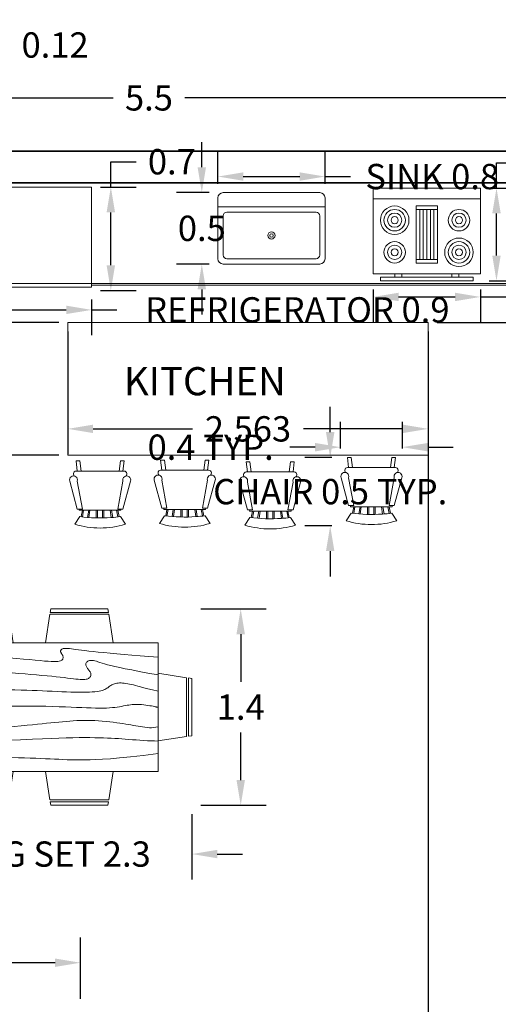
# Model space of a CAD drawing. Units: metres. Extents: x 4.8 to 18.3, y 28.2 to 89.8.
# Tile 3 of 4: x 8.6 to 12, y 36.6 to 43.6. Entities that reach past the tile are written whole.
import ezdxf

# ---------------------------------------------------------------- set-up
doc = ezdxf.new("R2010")
doc.units = ezdxf.units.M
doc.header["$MEASUREMENT"] = 0
doc.layers.get('Defpoints').update_dxf_attribs({"color": 3})
for name, color, linetype, lineweight in [('A-ANNO-DIMS', 2, 'Continuous', 18), ('A-AREA-IDEN', 7, 'Continuous', 25), ('A-EQPM', 8, 'Continuous', 18), ('A-FLOR-CASE', 8, 'Continuous', 18), ('A-FLOR-FIXT', 9, 'Continuous', 18), ('A-FURN', 8, 'Continuous', 18), ('A-WALL', 7, 'Continuous', 35)]:
    doc.layers.add(name, color=color, linetype=linetype, lineweight=lineweight)
doc.styles.get("Standard").update_dxf_attribs({"font": 'arial.ttf'})
doc.dimstyles.get("Standard").update_dxf_attribs({"dimtxt": 0.18, "dimasz": 0.18, "dimexe": 0.18, "dimexo": 0.0625, "dimgap": 0.09, "dimtad": 0, "dimtih": 1, "dimtoh": 1, "dimdec": 1, "dimzin": 0, "dimdsep": 46, "dimtxsty": 'Standard', "dimcen": 0.09, "dimadec": 0, "dimazin": 0, "dimtfac": 1, "dimtdec": 1, "dimtofl": 0, "dimtmove": 0, "dimatfit": 3, "dimfxl": 1, "dimtolj": 1, "dimtzin": 0, "dimarcsym": 0})

# ---------------------------------------------------------------- blocks, each defined once
blk = doc.blocks.new('Refrigerator-2 door - 36 in top')
for p, q in [((0, -26.999999), (36, -26.999999)), ((12, -26.999999), (12, -28.999999)), ((11, -27.999999), (11, -28.999999)), ((11, -28.999999), (13, -28.999999)), ((13, -28.999999), (13, -27.999999))]:
    blk.add_line(p, q)
blk.add_lwpolyline([(0, -27.999999), (0, 0), (36, 0), (36, -27.999999)], close=True)
blk = doc.blocks.new('Range-Oven - 30 in top')
for p, q in [((0, -3), (30, -3)), ((12, -6), (18, -6)), ((13, -20), (13, -6)), ((14, -6), (14, -20)), ((15, -20), (15, -6)), ((16, -6), (16, -20)), ((17, -20), (17, -6)), ((18, -20), (12, -20)), ((6, -24), (6, -25)), ((8, -25), (8, -24)), ((22, -25), (22, -24)), ((24, -24), (24, -25))]:
    blk.add_line(p, q)
for points in [[(0, -24), (0, 0), (30, 0), (30, -24)], [(12, -21), (12, -5), (18, -5), (18, -21)], [(2, -26), (2, -25), (28, -25), (28, -26)]]:
    blk.add_lwpolyline(points, close=True)
for centre, radius in [((6, -9), 4), ((6, -9), 3), ((6, -9), 2), ((6, -9), 1), ((24, -9), 3), ((24, -9), 2), ((24, -9), 1), ((6, -18), 3), ((6, -18), 2), ((24, -18), 4), ((24, -18), 3), ((24, -18), 2), ((6, -18), 1), ((24, -18), 1)]:
    blk.add_circle(centre, radius)
blk = doc.blocks.new('Sink-single - 30 in top')
blk.add_line((-15, -3.999996), (15, -3.999996))
for points in [[(-13.5, 0), (13.5, 0)], [(-15, -18.499996), (-15, -1.5)], [(15, -1.5), (15, -18.499996)], [(-12.5, -5.499996), (12.5, -5.499996)], [(-13.5, -17.499996), (-13.5, -6.499996)], [(13.5, -6.499996), (13.5, -17.499996)], [(12.5, -18.499996), (-12.5, -18.499996)], [(13.5, -19.999996), (-13.5, -19.999996)]]:
    blk.add_lwpolyline(points)
for radius in [1, 0.5]:
    blk.add_circle((0, -11.999996), radius)
for centre, radius, start, end in [((-13.5, -1.5), 1.5, 90, 180), ((13.5, -1.5), 1.5, 0, 90), ((-12.5, -6.499996), 1, 90, 180), ((12.5, -6.499996), 1, 0, 90), ((-13.5, -18.499996), 1.5, 180, 270), ((-12.5, -17.499996), 1, 180, 270), ((12.5, -17.499996), 1, 270, 0), ((13.5, -18.499996), 1.5, 270, 0)]:
    blk.add_arc(centre, radius, start, end)
blk = doc.blocks.new('Dining Set - 36 x 72 in.')
for p, q in [((-22.2343, 26.00059), (-23.4847, 17.99762)), ((-22.2304, 26), (-5.7608, 26)), ((-22, 27.5), (-22.1562, 26.50042)), ((-5.8416, 26.5), (-22.1534, 26.5)), ((-22, 27.5), (-6, 27.5)), ((-5.8437, 26.49966), (-6, 27.5)), ((-4.5152, 17.99762), (-5.7655, 25.99926)), ((5.7657, 26.00059), (4.5153, 17.99762)), ((5.7696, 26), (22.2392, 26)), ((6, 27.5), (5.8438, 26.50042)), ((22.1584, 26.5), (5.8466, 26.5)), ((6, 27.5), (22, 27.5)), ((22.1563, 26.49966), (22, 27.5)), ((23.4848, 17.99762), (22.2345, 25.99926)), ((36, 18), (-36, 18)), ((-36, 18), (-36, -18)), ((36, -18), (36, 18)), ((-44.0006, 8.23428), (-35.9976, 9.48474)), ((44.0006, 8.23428), (35.9976, 9.48474)), ((-45.5, 8), (-44.5004, 8.15617)), ((-45.5, 8), (-45.5, -8)), ((-44.5, -8.15843), (-44.5, 8.15338)), ((-44, 8.23041), (-44, -8.23915)), ((44, 8.23041), (44, -8.23915)), ((44.5, -8.15843), (44.5, 8.15338)), ((45.5, 8), (44.5005, 8.15617)), ((45.5, 8), (45.5, -8)), ((-44.4997, -8.15631), (-45.5, -8)), ((-35.9976, -9.48476), (-43.9993, -8.2345)), ((35.9976, -9.48476), (43.9993, -8.2345)), ((44.4997, -8.15631), (45.5, -8)), ((-36, -18), (36, -18)), ((-22.2343, -26.0006), (-23.4847, -17.99762)), ((-4.5152, -17.99762), (-5.7655, -25.99928)), ((5.7657, -26.0006), (4.5153, -17.99762)), ((23.4848, -17.99762), (22.2345, -25.99928)), ((-22.2304, -26), (-5.7608, -26)), ((-22, -27.5), (-22.1562, -26.50044)), ((-5.8416, -26.5), (-22.1534, -26.5)), ((-22, -27.5), (-6, -27.5)), ((-5.8437, -26.49967), (-6, -27.5)), ((5.7696, -26), (22.2392, -26)), ((6, -27.5), (5.8438, -26.50044)), ((22.1584, -26.5), (5.8466, -26.5)), ((6, -27.5), (22, -27.5)), ((22.1563, -26.49967), (22, -27.5))]:
    blk.add_line(p, q)
for points in [[(-36, 15), (-31.1772, 14.97754), (-26.8079, 14.91406), (-22.8538, 14.81543), (-19.276, 14.6875), (-16.0362, 14.53613), (-13.0957, 14.36718), (-10.4159, 14.18652), (-7.9583, 14), (-5.6904, 13.81315), (-3.6035, 13.63021), (-1.6954, 13.45508), (0.0365, 13.29166), (1.5945, 13.14388), (2.9811, 13.01562), (4.1988, 12.9108), (5.25, 12.83333), (6.1393, 12.78613), (6.8802, 12.76823), (7.4883, 12.77767), (7.9792, 12.8125), (8.3685, 12.87077), (8.6719, 12.95052), (8.9049, 13.0498), (9.0833, 13.16666), (9.2205, 13.29899), (9.3216, 13.44401), (9.3895, 13.59879), (9.4271, 13.76041), (9.4373, 13.92594), (9.4232, 14.09245), (9.3875, 14.257), (9.3333, 14.41666), (9.2638, 14.56917), (9.1836, 14.71484), (9.0975, 14.85465), (9.0104, 14.98958), (8.9272, 15.1206), (8.8529, 15.2487), (8.7922, 15.37483), (8.75, 15.5), (8.7305, 15.62467), (8.7344, 15.74739), (8.7617, 15.86621), (8.8125, 15.97916), (8.8867, 16.08431), (8.9844, 16.17968), (9.1055, 16.26334), (9.25, 16.33333), (9.4189, 16.38802), (9.6172, 16.42708), (9.8506, 16.45052), (10.125, 16.45833), (10.4463, 16.45052), (10.8203, 16.42708), (11.2529, 16.38802), (11.75, 16.33333), (12.3184, 16.26318), (12.9694, 16.17838), (13.7151, 16.07991), (14.5677, 15.96875), (15.5395, 15.84586), (16.6426, 15.71224), (17.8893, 15.56884), (19.2917, 15.41666), (20.859, 15.25667), (22.5879, 15.08984), (24.4721, 14.91715), (26.5052, 14.73958), (28.6809, 14.5581), (30.9929, 14.3737), (33.4347, 14.18733), (36, 14)], [(-36, 10), (-28.9766, 10.14274), (-23.1725, 10.20442), (-18.4241, 10.19775), (-14.5677, 10.13541), (-11.4399, 10.03011), (-8.877, 9.89453), (-6.7154, 9.74137), (-4.7917, 9.58333), (-2.9698, 9.43082), (-1.2246, 9.28515), (0.4415, 9.14534), (2.026, 9.01041), (3.5266, 8.87939), (4.9408, 8.7513), (6.266, 8.62516), (7.5, 8.5), (8.6411, 8.37549), (9.6914, 8.2539), (10.6538, 8.13818), (11.5312, 8.03125), (12.3267, 7.93603), (13.043, 7.85547), (13.6831, 7.79248), (14.25, 7.75), (14.7471, 7.7303), (15.1797, 7.73307), (15.5537, 7.75732), (15.875, 7.80208), (16.1494, 7.86637), (16.3828, 7.94922), (16.5811, 8.04964), (16.75, 8.16666), (16.8944, 8.29915), (17.0143, 8.44531), (17.1089, 8.60319), (17.1771, 8.77083), (17.218, 8.94629), (17.2305, 9.1276), (17.2137, 9.31282), (17.1667, 9.5), (17.0895, 9.6875), (16.987, 9.875), (16.8649, 10.0625), (16.7292, 10.25), (16.5856, 10.4375), (16.4401, 10.625), (16.2985, 10.8125), (16.1667, 11), (16.05, 11.18733), (15.9518, 11.3737), (15.8752, 11.5581), (15.8229, 11.73958), (15.798, 11.91715), (15.8034, 12.08984), (15.842, 12.25667), (15.9167, 12.41666), (16.0295, 12.56836), (16.1784, 12.70833), (16.3605, 12.83268), (16.5729, 12.9375), (16.8127, 13.01888), (17.0768, 13.07291), (17.3625, 13.0957), (17.6667, 13.08333), (17.9894, 13.03312), (18.3418, 12.94726), (18.7382, 12.82918), (19.1927, 12.68229), (19.7195, 12.51001), (20.3327, 12.31575), (21.0465, 12.10294), (21.875, 11.875), (22.8357, 11.63354), (23.959, 11.37304), (25.2786, 11.08618), (26.8282, 10.76562), (28.6414, 10.40405), (30.752, 9.99414), (33.1936, 9.52856), (36, 9)], [(-36, 5.5), (-30.7157, 5.3348), (-26.069, 5.20963), (-21.9946, 5.11767), (-18.4271, 5.05208), (-15.3009, 5.00602), (-12.5508, 4.97265), (-10.1112, 4.94515), (-7.9167, 4.91666), (-5.909, 4.88167), (-4.0586, 4.83984), (-2.3429, 4.79215), (-0.7396, 4.73958), (0.7739, 4.6831), (2.22, 4.6237), (3.6213, 4.56233), (5, 4.5), (6.373, 4.43782), (7.7344, 4.3776), (9.0723, 4.32129), (10.375, 4.27083), (11.6309, 4.22819), (12.8281, 4.19531), (13.9551, 4.17415), (15, 4.16666), (15.954, 4.17448), (16.819, 4.19791), (17.6001, 4.23698), (18.3021, 4.29166), (18.9299, 4.36198), (19.4883, 4.44791), (19.9823, 4.54948), (20.4167, 4.66666), (20.7969, 4.79899), (21.1302, 4.94401), (21.4245, 5.09879), (21.6875, 5.26041), (21.9271, 5.42594), (22.1511, 5.59245), (22.3672, 5.757), (22.5834, 5.91666), (22.8065, 6.06868), (23.0404, 6.21093), (23.2879, 6.34147), (23.5521, 6.45833), (23.8358, 6.55957), (24.142, 6.64323), (24.4735, 6.70735), (24.8334, 6.75), (25.2235, 6.76969), (25.642, 6.76692), (26.0858, 6.74267), (26.5521, 6.69791), (27.0379, 6.63362), (27.5404, 6.55078), (28.0565, 6.45036), (28.5834, 6.33333), (29.1242, 6.19987), (29.7071, 6.04687), (30.3661, 5.87044), (31.1354, 5.66666), (32.0493, 5.43164), (33.142, 5.16146), (34.4475, 4.85221), (36, 4.5)], [(-36, -1), (-30.7915, -0.6591), (-26.0195, -0.38216), (-21.6519, -0.16284), (-17.6563, 0.00521), (-14.0005, 0.12833), (-10.6523, 0.21289), (-7.5796, 0.26522), (-4.75, 0.29166), (-2.134, 0.29793), (0.2878, 0.28711), (2.5317, 0.26163), (4.6146, 0.22396), (6.5529, 0.17651), (8.3633, 0.12174), (10.0623, 0.06209), (11.6667, 0), (13.1899, -0.06201), (14.6341, -0.1211), (15.9982, -0.17432), (17.2813, -0.21875), (18.4823, -0.25147), (19.6003, -0.26953), (20.6343, -0.27002), (21.5834, -0.25), (22.4481, -0.20768), (23.2357, -0.14584), (23.9549, -0.06836), (24.6146, 0.02083), (25.2235, 0.11784), (25.7904, 0.21875), (26.3241, 0.31966), (26.8334, 0.41666), (27.3265, 0.50618), (27.8099, 0.58593), (28.2894, 0.65397), (28.7709, 0.70833), (29.2601, 0.74707), (29.763, 0.76823), (30.2855, 0.76985), (30.8334, 0.75), (31.4088, 0.70784), (31.9994, 0.64713), (32.589, 0.57275), (33.1615, 0.48958), (33.7008, 0.4025), (34.1908, 0.3164), (34.6153, 0.23616), (34.9584, 0.16666), (35.2099, 0.11165), (35.3848, 0.07031), (35.504, 0.04069), (35.5886, 0.02083), (35.6594, 0.00879), (35.7377, 0.0026), (35.8442, 0.00032), (36, 0)], [(-36, -6.5), (-27.1843, -6.31267), (-20.084, -6.1263), (-14.469, -5.9419), (-10.1094, -5.76042), (-6.7752, -5.58285), (-4.2363, -5.41016), (-2.2629, -5.24333), (-0.625, -5.08334), (0.8708, -4.93099), (2.2715, -4.78646), (3.5872, -4.64974), (4.8281, -4.52084), (6.0046, -4.39974), (7.127, -4.28646), (8.2053, -4.18099), (9.25, -4.08334), (10.2705, -3.99382), (11.2734, -3.91407), (12.2647, -3.84603), (13.25, -3.79167), (14.2354, -3.75293), (15.2266, -3.73177), (16.2295, -3.73015), (17.25, -3.75), (18.2912, -3.79248), (19.3451, -3.85547), (20.4009, -3.93604), (21.4479, -4.03125), (22.4754, -4.13819), (23.4727, -4.25391), (24.4289, -4.37549), (25.3334, -4.5), (26.1785, -4.62492), (26.9694, -4.74935), (27.7145, -4.87281), (28.4219, -4.99479), (29.1, -5.11483), (29.7572, -5.23242), (30.4016, -5.34709), (31.0417, -5.45834), (31.6837, -5.56437), (32.3262, -5.65821), (32.9658, -5.73153), (33.599, -5.77604), (34.2224, -5.78345), (34.8327, -5.74545), (35.4264, -5.65373), (36, -5.5)], [(-36, -10), (-26.4022, -9.81299), (-18.4675, -9.62891), (-11.9839, -9.45069), (-6.7396, -9.28125), (-2.5226, -9.12354), (0.8789, -8.98047), (3.6769, -8.85498), (6.0833, -8.75), (8.2767, -8.66765), (10.3021, -8.60677), (12.1712, -8.56543), (13.8958, -8.54167), (15.4876, -8.53353), (16.9583, -8.53907), (18.3197, -8.55632), (19.5834, -8.58334), (20.7616, -8.61841), (21.8685, -8.66081), (22.9188, -8.71004), (23.9271, -8.76563), (24.9081, -8.82707), (25.8763, -8.89388), (26.8465, -8.96558), (27.8334, -9.04167), (28.8474, -9.12118), (29.8828, -9.20117), (30.93, -9.27824), (31.9792, -9.34896), (33.0205, -9.40991), (34.0443, -9.45768), (35.0407, -9.48885), (36, -9.5)], [(-36, -14.5), (-30.0881, -14.33513), (-25.0332, -14.21224), (-20.7312, -14.12647), (-17.0781, -14.07292), (-13.97, -14.04671), (-11.3027, -14.04297), (-8.9724, -14.05681), (-6.875, -14.08334), (-4.9224, -14.11833), (-3.0905, -14.16016), (-1.3709, -14.20785), (0.2448, -14.26042), (1.7647, -14.3169), (3.1973, -14.3763), (4.5507, -14.43767), (5.8333, -14.5), (7.0554, -14.5621), (8.235, -14.62175), (9.3922, -14.67652), (10.5469, -14.72396), (11.7192, -14.76164), (12.929, -14.78711), (14.1965, -14.79794), (15.5417, -14.79167), (16.9933, -14.76424), (18.6152, -14.70508), (20.4804, -14.60197), (22.6615, -14.44271), (25.2312, -14.21509), (28.2624, -13.9069), (31.8277, -13.50594), (36, -13)]]:
    blk.add_lwpolyline(points)
blk = doc.blocks.new('Chair - Rocking')
for p, q in [((-8, -4.5), (-10, -1.5)), ((8, -4.5), (10, -1.5)), ((-9, -7.5), (-12, -18.49999)), ((-7, -7.5), (-9, -7.5)), ((-9, -18.49999), (-7, -7.5)), ((-8.23428, -6.99939), (-8.3093, -7.47958)), ((-8.23041, -7), (8.23915, -7)), ((-7.5, -4.5), (-7, -7)), ((-6.5, -7), (-7.02225, -4.43)), ((-4.5, -7), (-4.96674, -4.19951)), ((-4, -7), (-4.40532, -4.16272)), ((-1.5, -4.05012), (-1.5, -7)), ((-1, -7), (-1, -4.05012)), ((1, -7), (1, -4.04655)), ((1.5, -4.05012), (1.5, -7)), ((4, -7), (4.40187, -4.18694)), ((4.5, -7), (4.96761, -4.19437)), ((6.5, -7), (7, -4.4057)), ((7.5, -4.5), (7, -7)), ((7, -7.5), (9, -7.5)), ((9, -18.49999), (7, -7.5)), ((8.31071, -7.48854), (8.23449, -7.00073)), ((9, -7.5), (12, -18.49999)), ((-10.36644, -20.64523), (-10.5, -21.49999)), ((-9, -22.49999), (-9.5, -26.49999)), ((0, -22.49999), (-9.5, -22.49999)), ((-8, -26.49999), (-7.5, -22.49999)), ((0, -22.49999), (9.5, -22.49999)), ((8, -26.49999), (7.5, -22.49999)), ((9, -22.49999), (9.5, -26.49999)), ((10.5, -21.49999), (10.3575, -20.58798)), ((-9.5, -26.49999), (-8, -26.49999)), ((9.5, -26.49999), (8, -26.49999))]:
    blk.add_line(p, q)
for centre, radius, start, end in [((0, -34.08333), 34.08333, 72.93847, 107.0615), ((0, -68.25004), 64.25, 93.92211, 97.15267), ((0, -68.25004), 64.25, 82.84733, 93.92211), ((-10.5, -18.99999), 1.58114, 161.5651, 18.43495), ((10.5, -18.99999), 1.58114, 161.5651, 18.43495), ((-9.5, -21.49999), 1, 180, 270), ((9.5, -21.49999), 1, 270, 0)]:
    blk.add_arc(centre, radius, start, end)
blk = doc.blocks.new('*D22')
at = {"layer": 'A-ANNO-DIMS', "color": 0, "lineweight": -2, "transparency": 16777216}
for p, q in [((6.7935, 42.7258), (6.7935, 43.223)), ((12.2935, 42.7258), (12.2935, 43.223)), ((6.9735, 43.043), (9.289, 43.043)), ((12.1135, 43.043), (9.798, 43.043))]:
    blk.add_line(p, q, dxfattribs=at)
at = {"layer": 'A-ANNO-DIMS', "color": 0, "transparency": 16777216}
for points in [[(6.9735, 43.073), (6.9735, 43.013), (6.7935, 43.043)], [(12.1135, 43.073), (12.1135, 43.013), (12.2935, 43.043)]]:
    blk.add_solid(points, dxfattribs=at)
at = {"layer": 'Defpoints', "color": 0, "transparency": 16777216}
for p in [(12.2935, 43.043), (6.7935, 42.6633), (12.2935, 42.6633)]:
    blk.add_point(p, dxfattribs=at)
at = {"layer": 'A-ANNO-DIMS', "color": 0, "transparency": 16777216, "insert": (9.5435, 43.043), "char_height": 0.18, "attachment_point": 5}
blk.add_mtext('\\A1;5.5', dxfattribs=at)
blk = doc.blocks.new('*D26')
at = {"layer": 'A-ANNO-DIMS', "color": 0, "lineweight": -2, "transparency": 16777216}
for p, q in [((10.0337, 42.4316), (10.0337, 42.6634)), ((10.7957, 42.4316), (10.7957, 42.6634)), ((10.2137, 42.4834), (10.6157, 42.4834)), ((10.7957, 42.4834), (10.9757, 42.4834))]:
    blk.add_line(p, q, dxfattribs=at)
at = {"layer": 'A-ANNO-DIMS', "color": 0, "transparency": 16777216}
for points in [[(10.2137, 42.5134), (10.2137, 42.4534), (10.0337, 42.4834)], [(10.6157, 42.5134), (10.6157, 42.4534), (10.7957, 42.4834)]]:
    blk.add_solid(points, dxfattribs=at)
at = {"layer": 'Defpoints', "color": 0, "transparency": 16777216}
for p in [(10.7957, 42.4834), (10.0337, 42.3691), (10.7957, 42.3691)]:
    blk.add_point(p, dxfattribs=at)
at = {"layer": 'A-ANNO-DIMS', "color": 0, "transparency": 16777216, "insert": (11.5577, 42.4834), "char_height": 0.18, "attachment_point": 5}
blk.add_mtext('\\A1;SINK 0.8', dxfattribs=at)
blk = doc.blocks.new('*D27')
at = {"layer": 'A-ANNO-DIMS', "color": 0, "lineweight": -2, "transparency": 16777216}
for p, q in [((9.9194, 42.5491), (9.9194, 42.7291)), ((9.9712, 42.3691), (9.7394, 42.3691)), ((9.9712, 41.8611), (9.7394, 41.8611)), ((9.9194, 41.6811), (9.9194, 41.5011))]:
    blk.add_line(p, q, dxfattribs=at)
at = {"layer": 'A-ANNO-DIMS', "color": 0, "transparency": 16777216}
for points in [[(9.8894, 42.5491), (9.9494, 42.5491), (9.9194, 42.3691)], [(9.8894, 41.6811), (9.9494, 41.6811), (9.9194, 41.8611)]]:
    blk.add_solid(points, dxfattribs=at)
at = {"layer": 'Defpoints', "color": 0, "transparency": 16777216}
for p in [(9.9194, 42.3691), (10.0337, 42.3691), (10.0337, 41.8611)]:
    blk.add_point(p, dxfattribs=at)
at = {"layer": 'A-ANNO-DIMS', "color": 0, "transparency": 16777216, "insert": (9.9194, 42.1151), "char_height": 0.18, "attachment_point": 5}
blk.add_mtext('\\A1;0.5', dxfattribs=at)
blk = doc.blocks.new('*D30')
at = {"layer": 'A-ANNO-DIMS', "color": 0, "lineweight": -2, "transparency": 16777216}
for p, q in [((10.8323, 40.6653), (10.8323, 40.8453)), ((10.8428, 40.4853), (10.6523, 40.4853)), ((10.8428, 39.9989), (10.6523, 39.9989)), ((10.8323, 39.8189), (10.8323, 39.6389))]:
    blk.add_line(p, q, dxfattribs=at)
at = {"layer": 'A-ANNO-DIMS', "color": 0, "transparency": 16777216}
for points in [[(10.8023, 40.6653), (10.8623, 40.6653), (10.8323, 40.4853)], [(10.8023, 39.8189), (10.8623, 39.8189), (10.8323, 39.9989)]]:
    blk.add_solid(points, dxfattribs=at)
at = {"layer": 'Defpoints', "color": 0, "transparency": 16777216}
for p in [(10.9053, 40.4853), (10.8323, 39.9989), (10.9053, 39.9989)]:
    blk.add_point(p, dxfattribs=at)
at = {"layer": 'A-ANNO-DIMS', "color": 0, "transparency": 16777216, "insert": (10.8323, 40.2421), "char_height": 0.18, "attachment_point": 5}
blk.add_mtext('\\A1;CHAIR 0.5 TYP.', dxfattribs=at)
blk = doc.blocks.new('*D31')
at = {"layer": 'A-ANNO-DIMS', "color": 0, "lineweight": -2, "transparency": 16777216}
for p, q in [((10.9053, 40.5478), (10.9053, 40.7383)), ((11.3455, 40.5478), (11.3455, 40.7383)), ((10.7253, 40.5583), (10.5453, 40.5583)), ((11.5255, 40.5583), (11.7055, 40.5583))]:
    blk.add_line(p, q, dxfattribs=at)
at = {"layer": 'A-ANNO-DIMS', "color": 0, "transparency": 16777216}
for points in [[(10.7253, 40.5883), (10.7253, 40.5283), (10.9053, 40.5583)], [(11.5255, 40.5883), (11.5255, 40.5283), (11.3455, 40.5583)]]:
    blk.add_solid(points, dxfattribs=at)
at = {"layer": 'Defpoints', "color": 0, "transparency": 16777216}
for p in [(10.9053, 40.5583), (10.9053, 40.4853), (11.3455, 40.4853)]:
    blk.add_point(p, dxfattribs=at)
at = {"layer": 'A-ANNO-DIMS', "color": 0, "transparency": 16777216, "insert": (9.9823, 40.5583), "char_height": 0.18, "attachment_point": 5}
blk.add_mtext('\\A1;0.4 TYP.', dxfattribs=at)
blk = doc.blocks.new('*D36')
at = {"layer": 'A-ANNO-DIMS', "color": 0, "lineweight": -2, "transparency": 16777216}
for p, q in [((8.2211, 41.6097), (8.2211, 41.355)), ((9.1355, 41.6097), (9.1355, 41.355)), ((8.4011, 41.535), (8.9555, 41.535)), ((9.1355, 41.535), (9.3155, 41.535))]:
    blk.add_line(p, q, dxfattribs=at)
at = {"layer": 'A-ANNO-DIMS', "color": 0, "transparency": 16777216}
for points in [[(8.4011, 41.565), (8.4011, 41.505), (8.2211, 41.535)], [(8.9555, 41.565), (8.9555, 41.505), (9.1355, 41.535)]]:
    blk.add_solid(points, dxfattribs=at)
at = {"layer": 'Defpoints', "color": 0, "transparency": 16777216}
for p in [(8.2211, 41.6722), (9.1355, 41.6722), (9.1355, 41.535)]:
    blk.add_point(p, dxfattribs=at)
at = {"layer": 'A-ANNO-DIMS', "color": 0, "transparency": 16777216, "insert": (10.5987, 41.535), "char_height": 0.18, "attachment_point": 5}
blk.add_mtext('\\A1;REFRIGERATOR 0.9', dxfattribs=at)
blk = doc.blocks.new('*D37')
at = {"layer": 'A-ANNO-DIMS', "color": 0, "lineweight": -2, "transparency": 16777216}
for p, q in [((9.2726, 42.4088), (9.2726, 42.5888)), ((9.2726, 42.5888), (9.4526, 42.5888)), ((9.198, 42.4088), (9.4526, 42.4088)), ((9.2726, 41.8522), (9.2726, 42.2288)), ((9.198, 41.6722), (9.4526, 41.6722))]:
    blk.add_line(p, q, dxfattribs=at)
at = {"layer": 'A-ANNO-DIMS', "color": 0, "transparency": 16777216}
for points in [[(9.2426, 42.2288), (9.3026, 42.2288), (9.2726, 42.4088)], [(9.2426, 41.8522), (9.3026, 41.8522), (9.2726, 41.6722)]]:
    blk.add_solid(points, dxfattribs=at)
at = {"layer": 'Defpoints', "color": 0, "transparency": 16777216}
for p in [(9.1355, 42.4088), (9.2726, 42.4088), (9.1355, 41.6722)]:
    blk.add_point(p, dxfattribs=at)
at = {"layer": 'A-ANNO-DIMS', "color": 0, "transparency": 16777216, "insert": (9.7065, 42.5888), "char_height": 0.18, "attachment_point": 5}
blk.add_mtext('\\A1;0.7', dxfattribs=at)
blk = doc.blocks.new('*D38')
at = {"layer": 'A-ANNO-DIMS', "color": 0, "lineweight": -2, "transparency": 16777216}
for p, q in [((11.1383, 41.6788), (11.1383, 41.447)), ((11.9003, 41.6788), (11.9003, 41.447)), ((11.3183, 41.627), (11.7203, 41.627)), ((11.9003, 41.627), (12.0803, 41.627))]:
    blk.add_line(p, q, dxfattribs=at)
at = {"layer": 'A-ANNO-DIMS', "color": 0, "transparency": 16777216}
for points in [[(11.3183, 41.657), (11.3183, 41.597), (11.1383, 41.627)], [(11.7203, 41.657), (11.7203, 41.597), (11.9003, 41.627)]]:
    blk.add_solid(points, dxfattribs=at)
at = {"layer": 'Defpoints', "color": 0, "transparency": 16777216}
for p in [(11.1383, 41.7413), (11.9003, 41.7413), (11.9003, 41.627)]:
    blk.add_point(p, dxfattribs=at)
at = {"layer": 'A-ANNO-DIMS', "color": 0, "transparency": 16777216, "insert": (12.8117, 41.627), "char_height": 0.18, "attachment_point": 5}
blk.add_mtext('\\A1;RANGE 0.8', dxfattribs=at)
blk = doc.blocks.new('*D39')
at = {"layer": 'A-ANNO-DIMS', "color": 0, "lineweight": -2, "transparency": 16777216}
for p, q in [((12.0146, 42.4017), (12.0146, 42.5817)), ((12.0146, 42.5817), (12.1946, 42.5817)), ((11.9628, 42.4017), (12.1946, 42.4017)), ((12.0146, 41.9213), (12.0146, 42.2217)), ((11.9628, 41.7413), (12.1946, 41.7413))]:
    blk.add_line(p, q, dxfattribs=at)
at = {"layer": 'A-ANNO-DIMS', "color": 0, "transparency": 16777216}
for points in [[(11.9846, 42.2217), (12.0446, 42.2217), (12.0146, 42.4017)], [(11.9846, 41.9213), (12.0446, 41.9213), (12.0146, 41.7413)]]:
    blk.add_solid(points, dxfattribs=at)
at = {"layer": 'Defpoints', "color": 0, "transparency": 16777216}
for p in [(11.9003, 42.4017), (12.0146, 42.4017), (11.9003, 41.7413)]:
    blk.add_point(p, dxfattribs=at)
at = {"layer": 'A-ANNO-DIMS', "color": 0, "transparency": 16777216, "insert": (12.4485, 42.5817), "char_height": 0.18, "attachment_point": 5}
blk.add_mtext('\\A1;0.7', dxfattribs=at)
blk = doc.blocks.new('*D41')
at = {"layer": 'A-ANNO-DIMS', "color": 0, "lineweight": -2, "transparency": 16777216}
for p, q in [((8.1252, 36.6335), (8.1252, 37.071)), ((9.0565, 36.6335), (9.0565, 37.071)), ((8.1252, 36.891), (7.9452, 36.891)), ((8.8765, 36.891), (8.3052, 36.891))]:
    blk.add_line(p, q, dxfattribs=at)
at = {"layer": 'A-ANNO-DIMS', "color": 0, "transparency": 16777216}
for points in [[(8.3052, 36.921), (8.3052, 36.861), (8.1252, 36.891)], [(8.8765, 36.921), (8.8765, 36.861), (9.0565, 36.891)]]:
    blk.add_solid(points, dxfattribs=at)
at = {"layer": 'Defpoints', "color": 0, "transparency": 16777216}
for p in [(8.1252, 36.891), (8.1252, 36.571), (9.0565, 36.571)]:
    blk.add_point(p, dxfattribs=at)
at = {"layer": 'A-ANNO-DIMS', "color": 0, "transparency": 16777216, "insert": (7.6911, 36.891), "char_height": 0.18, "attachment_point": 5}
blk.add_mtext('\\A1;0.9', dxfattribs=at)
blk = doc.blocks.new('*D44')
at = {"layer": 'A-ANNO-DIMS', "color": 0, "lineweight": -2, "transparency": 16777216}
for p, q in [((7.5379, 37.9483), (7.5379, 37.4841)), ((9.8493, 37.9483), (9.8493, 37.4841)), ((7.3579, 37.6641), (7.1779, 37.6641)), ((10.0293, 37.6641), (10.2093, 37.6641))]:
    blk.add_line(p, q, dxfattribs=at)
at = {"layer": 'A-ANNO-DIMS', "color": 0, "transparency": 16777216}
for points in [[(7.3579, 37.6941), (7.3579, 37.6341), (7.5379, 37.6641)], [(10.0293, 37.6941), (10.0293, 37.6341), (9.8493, 37.6641)]]:
    blk.add_solid(points, dxfattribs=at)
at = {"layer": 'Defpoints', "color": 0, "transparency": 16777216}
for p in [(7.5379, 38.0108), (9.8493, 38.0108), (9.8493, 37.6641)]:
    blk.add_point(p, dxfattribs=at)
at = {"layer": 'A-ANNO-DIMS', "color": 0, "transparency": 16777216, "insert": (8.6936, 37.6641), "char_height": 0.18, "attachment_point": 5}
blk.add_mtext('\\A1;DINING SET 2.3', dxfattribs=at)
blk = doc.blocks.new('*D45')
at = {"layer": 'A-ANNO-DIMS', "color": 0, "lineweight": -2, "transparency": 16777216}
for p, q in [((9.9118, 39.4078), (10.376, 39.4078)), ((10.196, 39.2278), (10.196, 38.8897)), ((10.196, 38.1908), (10.196, 38.5289)), ((9.9118, 38.0108), (10.376, 38.0108))]:
    blk.add_line(p, q, dxfattribs=at)
at = {"layer": 'A-ANNO-DIMS', "color": 0, "transparency": 16777216}
for points in [[(10.166, 39.2278), (10.226, 39.2278), (10.196, 39.4078)], [(10.166, 38.1908), (10.226, 38.1908), (10.196, 38.0108)]]:
    blk.add_solid(points, dxfattribs=at)
at = {"layer": 'Defpoints', "color": 0, "transparency": 16777216}
for p in [(9.8493, 39.4078), (10.196, 39.4078), (9.8493, 38.0108)]:
    blk.add_point(p, dxfattribs=at)
at = {"layer": 'A-ANNO-DIMS', "color": 0, "transparency": 16777216, "insert": (10.196, 38.7093), "char_height": 0.18, "attachment_point": 5}
blk.add_mtext('\\A1;1.4', dxfattribs=at)
blk = doc.blocks.new('*D58')
at = {"layer": 'A-ANNO-DIMS', "color": 0, "lineweight": -2, "transparency": 16777216}
for p, q in [((8.9662, 41.3821), (8.9662, 40.5086)), ((11.5294, 41.3821), (11.5294, 40.5086)), ((9.1462, 40.6886), (9.8526, 40.6886)), ((11.3494, 40.6886), (10.6431, 40.6886))]:
    blk.add_line(p, q, dxfattribs=at)
at = {"layer": 'A-ANNO-DIMS', "color": 0, "transparency": 16777216}
for points in [[(9.1462, 40.7186), (9.1462, 40.6586), (8.9662, 40.6886)], [(11.3494, 40.7186), (11.3494, 40.6586), (11.5294, 40.6886)]]:
    blk.add_solid(points, dxfattribs=at)
at = {"layer": 'Defpoints', "color": 0, "transparency": 16777216}
for p in [(8.9662, 41.4446), (11.5294, 41.4446), (8.9662, 40.6886)]:
    blk.add_point(p, dxfattribs=at)
at = {"layer": 'A-ANNO-DIMS', "color": 0, "transparency": 16777216, "insert": (10.2478, 40.6886), "char_height": 0.18, "attachment_point": 5}
blk.add_mtext('\\A1;2.563', dxfattribs=at)
blk = doc.blocks.new('*D59')
at = {"layer": 'A-ANNO-DIMS', "color": 0, "lineweight": -2, "transparency": 16777216}
for p, q in [((8.9037, 41.4446), (5.8575, 41.4446)), ((6.0375, 41.2646), (6.0375, 41.1553)), ((6.0375, 40.6822), (6.0375, 40.7915)), ((8.9037, 40.5022), (5.8575, 40.5022))]:
    blk.add_line(p, q, dxfattribs=at)
at = {"layer": 'A-ANNO-DIMS', "color": 0, "transparency": 16777216}
for points in [[(6.0075, 41.2646), (6.0675, 41.2646), (6.0375, 41.4446)], [(6.0075, 40.6822), (6.0675, 40.6822), (6.0375, 40.5022)]]:
    blk.add_solid(points, dxfattribs=at)
at = {"layer": 'Defpoints', "color": 0, "transparency": 16777216}
for p in [(6.0375, 41.4446), (8.9662, 41.4446), (8.9662, 40.5022)]:
    blk.add_point(p, dxfattribs=at)
at = {"layer": 'A-ANNO-DIMS', "color": 0, "transparency": 16777216, "insert": (6.0375, 40.9734), "char_height": 0.18, "attachment_point": 5}
blk.add_mtext('\\A1;0.94', dxfattribs=at)
blk = doc.blocks.new('*D60')
at = {"layer": 'A-ANNO-DIMS', "color": 0, "lineweight": -2, "transparency": 16777216}
for p, q in [((12.1735, 41.6485), (12.1735, 29.7273)), ((11.5294, 41.3821), (11.5294, 29.7273)), ((11.7094, 29.9073), (11.9935, 29.9073)), ((12.1735, 29.9073), (12.3535, 29.9073))]:
    blk.add_line(p, q, dxfattribs=at)
at = {"layer": 'A-ANNO-DIMS', "color": 0, "transparency": 16777216}
for points in [[(11.7094, 29.9372), (11.7094, 29.8773), (11.5294, 29.9073)], [(11.9935, 29.9372), (11.9935, 29.8773), (12.1735, 29.9073)]]:
    blk.add_solid(points, dxfattribs=at)
at = {"layer": 'Defpoints', "color": 0, "transparency": 16777216}
for p in [(12.1735, 41.711), (11.5294, 41.4446), (12.1735, 29.9073)]:
    blk.add_point(p, dxfattribs=at)
at = {"layer": 'A-ANNO-DIMS', "color": 0, "transparency": 16777216, "insert": (12.7468, 29.9073), "char_height": 0.18, "attachment_point": 5}
blk.add_mtext('\\A1;0.644', dxfattribs=at)
blk = doc.blocks.new('*D61')
at = {"layer": 'A-ANNO-DIMS', "color": 0, "lineweight": -2, "transparency": 16777216}
for p, q in [((17.5495, 41.891), (17.5495, 42.071)), ((17.5495, 42.071), (17.7295, 42.071)), ((12.236, 41.711), (17.7295, 41.711)), ((11.5919, 41.4446), (17.7295, 41.4446)), ((17.5495, 41.2646), (17.5495, 41.0846))]:
    blk.add_line(p, q, dxfattribs=at)
at = {"layer": 'A-ANNO-DIMS', "color": 0, "transparency": 16777216}
for points in [[(17.5195, 41.891), (17.5795, 41.891), (17.5495, 41.711)], [(17.5195, 41.2646), (17.5795, 41.2646), (17.5495, 41.4446)]]:
    blk.add_solid(points, dxfattribs=at)
at = {"layer": 'Defpoints', "color": 0, "transparency": 16777216}
for p in [(12.1735, 41.711), (17.5495, 41.711), (11.5294, 41.4446)]:
    blk.add_point(p, dxfattribs=at)
at = {"layer": 'A-ANNO-DIMS', "color": 0, "transparency": 16777216, "insert": (18.0533, 42.071), "char_height": 0.18, "attachment_point": 5}
blk.add_mtext('\\A1;0.27', dxfattribs=at)
blk = doc.blocks.new('*D63')
at = {"layer": 'A-ANNO-DIMS', "color": 0, "lineweight": -2, "transparency": 16777216}
for p, q in [((8.0735, 42.5007), (8.0735, 43.5992)), ((8.1935, 42.5007), (8.1935, 43.5992)), ((7.8935, 43.4192), (7.7135, 43.4192)), ((8.3735, 43.4192), (8.5535, 43.4192))]:
    blk.add_line(p, q, dxfattribs=at)
at = {"layer": 'A-ANNO-DIMS', "color": 0, "transparency": 16777216}
for points in [[(7.8935, 43.4492), (7.8935, 43.3892), (8.0735, 43.4192)], [(8.3735, 43.4492), (8.3735, 43.3892), (8.1935, 43.4192)]]:
    blk.add_solid(points, dxfattribs=at)
at = {"layer": 'Defpoints', "color": 0, "transparency": 16777216}
for p in [(8.1935, 43.4192), (8.0735, 42.4382), (8.1935, 42.4382)]:
    blk.add_point(p, dxfattribs=at)
at = {"layer": 'A-ANNO-DIMS', "color": 0, "transparency": 16777216, "insert": (8.8763, 43.4192), "char_height": 0.18, "attachment_point": 5}
blk.add_mtext('\\A1;0.12', dxfattribs=at)

msp = doc.modelspace()

# ---------------------------------------------------------------- linework, layer by layer
at = {"layer": 'A-FLOR-CASE'}
for p, q in [((9.1355, 41.723), (12.1735, 41.723)), ((9.1355, 41.711), (12.1735, 41.711))]:
    msp.add_line(p, q, dxfattribs=at)
msp.add_lwpolyline([(8.9662, 41.4446), (11.5294, 41.4446), (11.5294, 40.5022), (8.9662, 40.5022)], close=True, dxfattribs=at)
at = {"layer": 'A-WALL'}
for p, q in [((6.7935, 42.6633), (14.7935, 42.6633)), ((8.1935, 42.4382), (12.1735, 42.4382))]:
    msp.add_line(p, q, dxfattribs=at)

# ---------------------------------------------------------------- block references
at = {"layer": 'A-EQPM', "xscale": 0.0254, "yscale": 0.0254, "zscale": 0.0254}
for name, p in [('Refrigerator-2 door - 36 in top', (8.2211, 42.4088)), ('Range-Oven - 30 in top', (11.1383, 42.4017))]:
    msp.add_blockref(name, p, dxfattribs=at)
at = {"layer": 'A-FLOR-FIXT', "xscale": 0.0254, "yscale": 0.0254, "zscale": 0.0254}
msp.add_blockref('Sink-single - 30 in top', (10.4147, 42.3691), dxfattribs=at)
at = {"layer": 'A-FURN', "xscale": 0.0180162715215053, "yscale": 0.0180162715215053, "zscale": 0.0180162715215053, "rotation": 180}
for p in [(11.1254, 40.0079), (9.1963, 39.9831), (9.798, 39.9893), (10.4059, 39.9769)]:
    msp.add_blockref('Chair - Rocking', p, dxfattribs=at)
at = {"layer": 'A-FURN', "xscale": 0.0254, "yscale": 0.0254, "zscale": 0.0254}
msp.add_blockref('Dining Set - 36 x 72 in.', (8.6936, 38.7093), dxfattribs=at)

# ---------------------------------------------------------------- texts
at = {"layer": 'A-AREA-IDEN', "insert": (9.3659, 41.1277), "char_height": 0.2, "attachment_point": 1}
msp.add_mtext_dynamic_manual_height_columns('KITCHEN', width=0.479061, gutter_width=1, heights=[0], dxfattribs=at)

# ---------------------------------------------------------------- dimensions: what is measured, and where the dimension line sits
at = {"layer": 'A-ANNO-DIMS'}
for base, p1, p2, override, picture, middle in [((8.1935, 43.4192), (8.0735, 42.4382), (8.1935, 42.4382), {"dimdec": 2, "dimlfac": 1, "dimrnd": 0, "dimzin": 0, "dimdsep": 46, "dimlunit": 2}, '*D63', (8.8763, 43.4192)), ((12.2935, 43.043), (6.7935, 42.6633), (12.2935, 42.6633), {"dimclrd": 0, "dimclre": 0, "dimclrt": 0}, '*D22', (9.5435, 43.043)), ((12.1735, 29.9073), (11.5294, 41.4446), (12.1735, 41.711), {"dimdec": 3, "dimlfac": 1, "dimrnd": 0, "dimzin": 0, "dimdsep": 46, "dimlunit": 2}, '*D60', (12.7468, 29.9073))]:
    dim = msp.add_linear_dim(base=base, p1=p1, p2=p2, dimstyle='Standard', override=override, dxfattribs=at)
    dim.commit()
    dim.dimension.update_dxf_attribs({"geometry": picture, "text_midpoint": middle})
for base, p1, p2, angle, override, picture, middle in [((9.9194, 42.3691), (10.0337, 41.8611), (10.0337, 42.3691), 90, {"dimdec": 1, "dimlfac": 1, "dimrnd": 0, "dimzin": 0, "dimdsep": 46, "dimlunit": 2}, '*D27', (9.9194, 42.1151)), ((9.2726, 42.4088), (9.1355, 41.6722), (9.1355, 42.4088), 90, {"dimdec": 1, "dimlfac": 1, "dimrnd": 0, "dimzin": 0, "dimdsep": 46, "dimlunit": 2}, '*D37', (9.7065, 42.5888)), ((12.0146, 42.4017), (11.9003, 41.7413), (11.9003, 42.4017), 90, {"dimdec": 1, "dimlfac": 1, "dimrnd": 0, "dimzin": 0, "dimdsep": 46, "dimlunit": 2}, '*D39', (12.4485, 42.5817)), ((17.5495, 41.711), (11.5294, 41.4446), (12.1735, 41.711), 90, {"dimdec": 2, "dimlfac": 1, "dimrnd": 0, "dimzin": 0, "dimdsep": 46, "dimlunit": 2}, '*D61', (18.0533, 42.071)), ((6.0375, 41.4446), (8.9662, 40.5022), (8.9662, 41.4446), 90, {"dimdec": 2, "dimlfac": 1, "dimrnd": 0, "dimzin": 0, "dimdsep": 46, "dimlunit": 2}, '*D59', (6.0375, 40.9734)), ((8.9662, 40.6886), (11.5294, 41.4446), (8.9662, 41.4446), 180, {"dimdec": 3, "dimlfac": 1, "dimrnd": 0, "dimzin": 0, "dimdsep": 46, "dimlunit": 2}, '*D58', (10.2478, 40.6886)), ((10.196, 39.4078), (9.8493, 38.0108), (9.8493, 39.4078), 90, {"dimdec": 1, "dimlfac": 1, "dimrnd": 0, "dimzin": 0, "dimdsep": 46, "dimlunit": 2}, '*D45', (10.196, 38.7093)), ((8.1252, 36.891), (9.0565, 36.571), (8.1252, 36.571), 180, {"dimdec": 1, "dimlfac": 1, "dimrnd": 0, "dimzin": 0, "dimdsep": 46, "dimlunit": 2}, '*D41', (7.6911, 36.891))]:
    dim = msp.add_linear_dim(base=base, p1=p1, p2=p2, angle=angle, dimstyle='Standard', override=override, dxfattribs=at)
    dim.commit()
    dim.dimension.update_dxf_attribs({"geometry": picture, "text_midpoint": middle})
for base, p1, p2, text, picture, middle in [((10.7957, 42.4834), (10.0337, 42.3691), (10.7957, 42.3691), 'SINK <>', '*D26', (11.5577, 42.4834)), ((11.9003, 41.627), (11.1383, 41.7413), (11.9003, 41.7413), 'RANGE <>', '*D38', (12.8117, 41.627)), ((9.1355, 41.535), (8.2211, 41.6722), (9.1355, 41.6722), 'REFRIGERATOR <>', '*D36', (10.5987, 41.535)), ((9.8493, 37.6641), (7.5379, 38.0108), (9.8493, 38.0108), 'DINING SET <>', '*D44', (8.6936, 37.6641))]:
    dim = msp.add_linear_dim(base=base, p1=p1, p2=p2, text=text, dimstyle='Standard', override={"dimdec": 1, "dimlfac": 1, "dimrnd": 0, "dimzin": 0, "dimdsep": 46, "dimlunit": 2}, dxfattribs=at)
    dim.commit()
    dim.dimension.update_dxf_attribs({"geometry": picture, "text_midpoint": middle})
for base, p1, p2, angle, text, picture, middle in [((10.8323, 39.9989), (10.9053, 40.4853), (10.9053, 39.9989), 270, 'CHAIR <> TYP.', '*D30', (10.8323, 40.2421)), ((10.9053, 40.5583), (11.3455, 40.4853), (10.9053, 40.4853), 180, '<> TYP.', '*D31', (9.9823, 40.5583))]:
    dim = msp.add_linear_dim(base=base, p1=p1, p2=p2, angle=angle, text=text, dimstyle='Standard', override={"dimdec": 1, "dimlfac": 1, "dimrnd": 0, "dimzin": 0, "dimdsep": 46, "dimlunit": 2}, dxfattribs=at)
    dim.commit()
    dim.dimension.update_dxf_attribs({"geometry": picture, "text_midpoint": middle})

doc.saveas('drawing.dxf')
